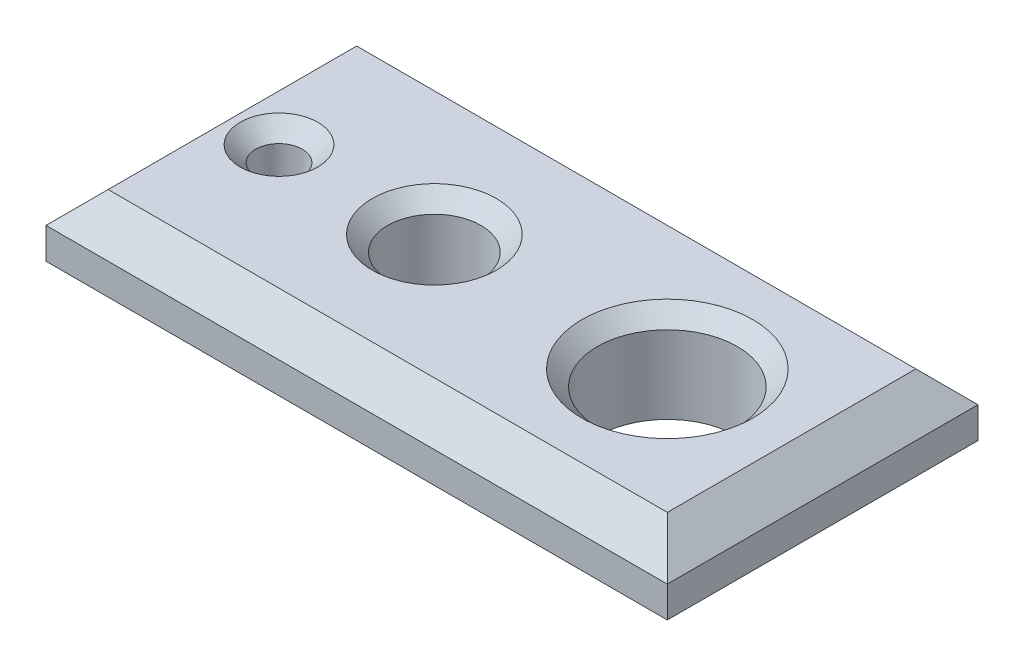
SolidWorks part; units mm, degrees
material "Plain Carbon Steel"
ref_plane "Front Plane" through (0, 0, 0) normal (0, 0, 1) x (1, 0, 0)
ref_plane "Top Plane" through (0, 0, 0) normal (0, 1, 0) x (1, 0, 0)
ref_plane "Right Plane" through (0, 0, 0) normal (1, 0, 0) x (0, 0, -1)
sketch "Base Plate Sketch" plane through (0, 0, 0) normal (0, 1, 0) x (1, 0, 0)
  line L1 (-100, -50) -> (100, -50)
  line L2 (-100, -50) -> (-100, 50)
  line L3 (-100, 50) -> (100, 50)
  line L4 (100, -50) -> (100, 50)
  line L5 (-100, -50) -> (100, 50) construction
  line L6 (-100, 50) -> (100, -50) construction
  point P0 (0, 0)
  dimension "D1" = 200
  dimension "D2" = 100
extrude "Base Plate 200x100x30" add sketch "Base Plate Sketch" along normal mid plane 30
chamfer "Plate End Chamfers 10mm" distance 10 angle 45 8 edges at (0, -15, -50) (-100, -15, 0) (0, -15, 50) (100, -15, 0) (0, 15, -50) (100, 15, 0) (0, 15, 50) (-100, 15, 0)
sketch "Pin Holes Sketch" plane through (0, 15, 0) normal (0, 1, 0) x (1, 0, 0)
  line L0 (-100, -50) -> (-100, 50) construction
  circle A0 centre (-75, 0) radius 7.5
  circle A1 centre (-25, 0) radius 15
  circle A2 centre (50, 0) radius 22.5
  dimension "D1" = 15
  dimension "D2" = 30
  dimension "D3" = 45
  dimension "D4" = 25
  dimension "D5" = 50
  dimension "D6" = 75
extrude "Pin Holes Ø15 Ø30 Ø45" cut sketch "Pin Holes Sketch" against normal up to surface (30 mm away) up to face at (0, -15, 0)
chamfer "Pin Hole Chamfers 5mm" distance 5 angle 45 3 edges at (50, 15, 22.5) (-25, 15, 15) (-75, 15, 7.5)
